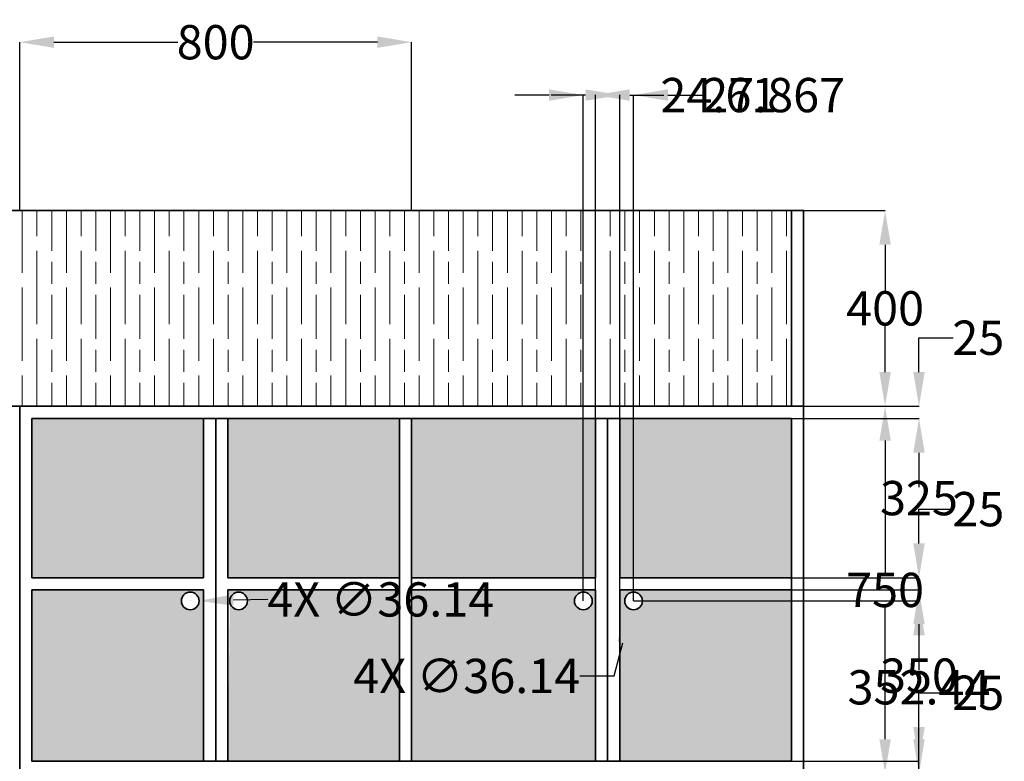
# Model space of a CAD drawing. Units: inches. Extents: x 600 to 5582, y -464 to 3142.
# Tile 9 of 9: x 3385 to 5394, y 1627 to 3142. Entities that reach past the tile are written whole.
import ezdxf

# ---------------------------------------------------------------- set-up
doc = ezdxf.new("R2010")
doc.units = ezdxf.units.IN
doc.header["$MEASUREMENT"] = 0
for name, color, linetype, lineweight in [('A-ANNO-DIMS', 2, 'Continuous', 18), ('A-ELEV', 7, 'Continuous', 35), ('A-ELEV-PATT', 252, 'Continuous', 13)]:
    doc.layers.add(name, color=color, linetype=linetype, lineweight=lineweight)
doc.styles.get("Standard").update_dxf_attribs({"font": 'arial.ttf'})
doc.dimstyles.get("Standard").update_dxf_attribs({"dimtxt": 70, "dimasz": 70, "dimexe": 0.18, "dimexo": 0.0625, "dimgap": 0.09, "dimtad": 0, "dimtih": 1, "dimtoh": 1, "dimdec": 0, "dimzin": 0, "dimdsep": 46, "dimtxsty": 'Standard', "dimcen": 0.09, "dimadec": 0, "dimazin": 0, "dimtfac": 1, "dimtdec": 0, "dimtofl": 0, "dimtmove": 0, "dimatfit": 3, "dimfxl": 1, "dimtolj": 1, "dimtzin": 0, "dimarcsym": 0})

# ---------------------------------------------------------------- blocks, each defined once
blk = doc.blocks.new('*D5')
at = {"layer": 'A-ANNO-DIMS', "color": 0, "lineweight": -2, "transparency": 16777216}
for p, q in [((4984.8, 2352.4), (5151.2, 2352.4)), ((5151, 2282.4), (5151, 2013.3)), ((5151, 1672.4), (5151, 1941.6)), ((4984.8, 1602.4), (5151.2, 1602.4))]:
    blk.add_line(p, q, dxfattribs=at)
at = {"layer": 'A-ANNO-DIMS', "color": 0, "transparency": 16777216}
for points in [[(5139.4, 2282.4), (5162.7, 2282.4), (5151, 2352.4)], [(5139.4, 1672.4), (5162.7, 1672.4), (5151, 1602.4)]]:
    blk.add_solid(points, dxfattribs=at)
at = {"layer": 'Defpoints', "color": 0, "transparency": 16777216}
for p in [(4984.7, 2352.4), (4984.7, 1602.4), (5151, 1602.4)]:
    blk.add_point(p, dxfattribs=at)
at = {"layer": 'A-ANNO-DIMS', "color": 0, "transparency": 16777216, "insert": (5151, 1977.4), "char_height": 70, "attachment_point": 5}
blk.add_mtext('\\A1;750', dxfattribs=at)
blk = doc.blocks.new('*D6')
at = {"layer": 'A-ANNO-DIMS', "color": 0, "lineweight": -2, "transparency": 16777216}
for p, q in [((4984.8, 2752.4), (5151.2, 2752.4)), ((5151, 2682.4), (5151, 2588.3)), ((5151, 2422.4), (5151, 2516.6)), ((4984.8, 2352.4), (5151.2, 2352.4))]:
    blk.add_line(p, q, dxfattribs=at)
at = {"layer": 'A-ANNO-DIMS', "color": 0, "transparency": 16777216}
for points in [[(5139.4, 2682.4), (5162.7, 2682.4), (5151, 2752.4)], [(5139.4, 2422.4), (5162.7, 2422.4), (5151, 2352.4)]]:
    blk.add_solid(points, dxfattribs=at)
at = {"layer": 'Defpoints', "color": 0, "transparency": 16777216}
for p in [(4984.7, 2752.4), (4984.7, 2352.4), (5151, 2352.4)]:
    blk.add_point(p, dxfattribs=at)
at = {"layer": 'A-ANNO-DIMS', "color": 0, "transparency": 16777216, "insert": (5151, 2552.4), "char_height": 70, "attachment_point": 5}
blk.add_mtext('\\A1;400', dxfattribs=at)
blk = doc.blocks.new('*D9')
at = {"layer": 'A-ANNO-DIMS', "color": 0, "lineweight": -2, "transparency": 16777216}
for p, q in [((3384.7, 2752.5), (3384.7, 3096.1)), ((3454.7, 3095.9), (3707.4, 3095.9)), ((4114.7, 3095.9), (3862.1, 3095.9)), ((4184.7, 2752.5), (4184.7, 3096.1))]:
    blk.add_line(p, q, dxfattribs=at)
at = {"layer": 'A-ANNO-DIMS', "color": 0, "transparency": 16777216}
for points in [[(3454.7, 3107.6), (3454.7, 3084.3), (3384.7, 3095.9)], [(4114.7, 3107.6), (4114.7, 3084.3), (4184.7, 3095.9)]]:
    blk.add_solid(points, dxfattribs=at)
at = {"layer": 'Defpoints', "color": 0, "transparency": 16777216}
for p in [(4184.7, 3095.9), (3384.7, 2752.4), (4184.7, 2752.4)]:
    blk.add_point(p, dxfattribs=at)
at = {"layer": 'A-ANNO-DIMS', "color": 0, "transparency": 16777216, "insert": (3784.7, 3095.9), "char_height": 70, "attachment_point": 5}
blk.add_mtext('\\A1;800', dxfattribs=at)
blk = doc.blocks.new('*D35')
at = {"layer": 'A-ANNO-DIMS', "color": 0, "lineweight": -2, "transparency": 16777216}
for p, q in [((5220.2, 1697.4), (5220.2, 1767.4)), ((5220.2, 1767.4), (5290.2, 1767.4)), ((4959.8, 1627.4), (5220.4, 1627.4)), ((4984.8, 1602.4), (5220.4, 1602.4)), ((5220.2, 1532.4), (5220.2, 1462.4))]:
    blk.add_line(p, q, dxfattribs=at)
at = {"layer": 'A-ANNO-DIMS', "color": 0, "transparency": 16777216}
for points in [[(5208.6, 1697.4), (5231.9, 1697.4), (5220.2, 1627.4)], [(5208.6, 1532.4), (5231.9, 1532.4), (5220.2, 1602.4)]]:
    blk.add_solid(points, dxfattribs=at)
at = {"layer": 'Defpoints', "color": 0, "transparency": 16777216}
for p in [(4959.7, 1627.4), (5220.2, 1627.4), (4984.7, 1602.4)]:
    blk.add_point(p, dxfattribs=at)
at = {"layer": 'A-ANNO-DIMS', "color": 0, "transparency": 16777216, "insert": (5341.3, 1767.4), "char_height": 70, "attachment_point": 5}
blk.add_mtext('\\A1;25', dxfattribs=at)
blk = doc.blocks.new('*D36')
at = {"layer": 'A-ANNO-DIMS', "color": 0, "lineweight": -2, "transparency": 16777216}
for p, q in [((4959.8, 1977.4), (5220.4, 1977.4)), ((5220.2, 1907.4), (5220.2, 1838.3)), ((5220.2, 1697.4), (5220.2, 1766.6)), ((4959.8, 1627.4), (5220.4, 1627.4))]:
    blk.add_line(p, q, dxfattribs=at)
at = {"layer": 'A-ANNO-DIMS', "color": 0, "transparency": 16777216}
for points in [[(5208.6, 1907.4), (5231.9, 1907.4), (5220.2, 1977.4)], [(5208.6, 1697.4), (5231.9, 1697.4), (5220.2, 1627.4)]]:
    blk.add_solid(points, dxfattribs=at)
at = {"layer": 'Defpoints', "color": 0, "transparency": 16777216}
for p in [(4959.7, 1977.4), (5220.2, 1977.4), (4959.7, 1627.4)]:
    blk.add_point(p, dxfattribs=at)
at = {"layer": 'A-ANNO-DIMS', "color": 0, "transparency": 16777216, "insert": (5220.2, 1802.4), "char_height": 70, "attachment_point": 5}
blk.add_mtext('\\A1;350', dxfattribs=at)
blk = doc.blocks.new('*D37')
at = {"layer": 'A-ANNO-DIMS', "color": 0, "lineweight": -2, "transparency": 16777216}
for p, q in [((5220.2, 2072.4), (5220.2, 2142.4)), ((5220.2, 2142.4), (5290.2, 2142.4)), ((4959.8, 2002.4), (5220.4, 2002.4)), ((4959.8, 1977.4), (5220.4, 1977.4)), ((5220.2, 1907.4), (5220.2, 1837.4))]:
    blk.add_line(p, q, dxfattribs=at)
at = {"layer": 'A-ANNO-DIMS', "color": 0, "transparency": 16777216}
for points in [[(5208.6, 2072.4), (5231.9, 2072.4), (5220.2, 2002.4)], [(5208.6, 1907.4), (5231.9, 1907.4), (5220.2, 1977.4)]]:
    blk.add_solid(points, dxfattribs=at)
at = {"layer": 'Defpoints', "color": 0, "transparency": 16777216}
for p in [(4959.7, 2002.4), (5220.2, 2002.4), (4959.7, 1977.4)]:
    blk.add_point(p, dxfattribs=at)
at = {"layer": 'A-ANNO-DIMS', "color": 0, "transparency": 16777216, "insert": (5341.3, 2142.4), "char_height": 70, "attachment_point": 5}
blk.add_mtext('\\A1;25', dxfattribs=at)
blk = doc.blocks.new('*D38')
at = {"layer": 'A-ANNO-DIMS', "color": 0, "lineweight": -2, "transparency": 16777216}
for p, q in [((4959.8, 2327.4), (5220.4, 2327.4)), ((5220.2, 2257.4), (5220.2, 2200.8)), ((5220.2, 2072.4), (5220.2, 2129.1)), ((4959.8, 2002.4), (5220.4, 2002.4))]:
    blk.add_line(p, q, dxfattribs=at)
at = {"layer": 'A-ANNO-DIMS', "color": 0, "transparency": 16777216}
for points in [[(5208.6, 2257.4), (5231.9, 2257.4), (5220.2, 2327.4)], [(5208.6, 2072.4), (5231.9, 2072.4), (5220.2, 2002.4)]]:
    blk.add_solid(points, dxfattribs=at)
at = {"layer": 'Defpoints', "color": 0, "transparency": 16777216}
for p in [(4959.7, 2327.4), (5220.2, 2327.4), (4959.7, 2002.4)]:
    blk.add_point(p, dxfattribs=at)
at = {"layer": 'A-ANNO-DIMS', "color": 0, "transparency": 16777216, "insert": (5220.2, 2164.9), "char_height": 70, "attachment_point": 5}
blk.add_mtext('\\A1;325', dxfattribs=at)
blk = doc.blocks.new('*D39')
at = {"layer": 'A-ANNO-DIMS', "color": 0, "lineweight": -2, "transparency": 16777216}
for p, q in [((5220.2, 2422.4), (5220.2, 2492.4)), ((5220.2, 2492.4), (5290.2, 2492.4)), ((4984.8, 2352.4), (5220.4, 2352.4)), ((4959.8, 2327.4), (5220.4, 2327.4)), ((5220.2, 2257.4), (5220.2, 2187.4))]:
    blk.add_line(p, q, dxfattribs=at)
at = {"layer": 'A-ANNO-DIMS', "color": 0, "transparency": 16777216}
for points in [[(5208.6, 2422.4), (5231.9, 2422.4), (5220.2, 2352.4)], [(5208.6, 2257.4), (5231.9, 2257.4), (5220.2, 2327.4)]]:
    blk.add_solid(points, dxfattribs=at)
at = {"layer": 'Defpoints', "color": 0, "transparency": 16777216}
for p in [(4984.7, 2352.4), (5220.2, 2352.4), (4959.7, 2327.4)]:
    blk.add_point(p, dxfattribs=at)
at = {"layer": 'A-ANNO-DIMS', "color": 0, "transparency": 16777216, "insert": (5341.3, 2492.4), "char_height": 70, "attachment_point": 5}
blk.add_mtext('\\A1;25', dxfattribs=at)
blk = doc.blocks.new('*D58')
at = {"layer": 'A-ANNO-DIMS', "color": 0, "lineweight": -2, "transparency": 16777216}
for p, q in [((3732.7, 1954.9), (3732.9, 1954.9)), ((3732.8, 1954.8), (3732.8, 1954.9)), ((3890.9, 1958), (3820.9, 1956.6))]:
    blk.add_line(p, q, dxfattribs=at)
at = {"layer": 'A-ANNO-DIMS', "color": 0, "transparency": 16777216}
blk.add_solid([(3820.6, 1968.3), (3821.1, 1944.9), (3750.9, 1955.2)], dxfattribs=at)
at = {"layer": 'Defpoints', "color": 0, "transparency": 16777216}
for p in [(3714.8, 1954.5), (3750.9, 1955.2)]:
    blk.add_point(p, dxfattribs=at)
at = {"layer": 'A-ANNO-DIMS', "color": 0, "transparency": 16777216, "insert": (4121.7, 1958), "char_height": 70, "attachment_point": 5}
blk.add_mtext('\\A1;4X ∅36.14', dxfattribs=at)
blk = doc.blocks.new('*D60')
at = {"layer": 'A-ANNO-DIMS', "color": 0, "lineweight": -2, "transparency": 16777216}
for p, q in [((4539.7, 2987.9), (4469.7, 2987.9)), ((4609.7, 1977.5), (4609.7, 2988.1)), ((4637.6, 1954.9), (4637.6, 2988.1)), ((4707.6, 2987.9), (4777.6, 2987.9))]:
    blk.add_line(p, q, dxfattribs=at)
at = {"layer": 'A-ANNO-DIMS', "color": 0, "transparency": 16777216}
for points in [[(4539.7, 2999.6), (4539.7, 2976.3), (4609.7, 2987.9)], [(4707.6, 2999.6), (4707.6, 2976.3), (4637.6, 2987.9)]]:
    blk.add_solid(points, dxfattribs=at)
at = {"layer": 'Defpoints', "color": 0, "transparency": 16777216}
for p in [(4637.6, 2987.9), (4609.7, 1977.4), (4637.6, 1954.9)]:
    blk.add_point(p, dxfattribs=at)
at = {"layer": 'A-ANNO-DIMS', "color": 0, "transparency": 16777216, "insert": (4923.6, 2987.9), "char_height": 70, "attachment_point": 5}
blk.add_mtext('\\A1;27.867', dxfattribs=at)
blk = doc.blocks.new('*D61')
at = {"layer": 'A-ANNO-DIMS', "color": 0, "lineweight": -2, "transparency": 16777216}
for p, q in [((4637.7, 1954.9), (5220.4, 1954.9)), ((5220.2, 1884.9), (5220.2, 1814.5)), ((5220.2, 1672.4), (5220.2, 1742.8)), ((4984.8, 1602.4), (5220.4, 1602.4))]:
    blk.add_line(p, q, dxfattribs=at)
at = {"layer": 'A-ANNO-DIMS', "color": 0, "transparency": 16777216}
for points in [[(5208.6, 1884.9), (5231.9, 1884.9), (5220.2, 1954.9)], [(5208.6, 1672.4), (5231.9, 1672.4), (5220.2, 1602.4)]]:
    blk.add_solid(points, dxfattribs=at)
at = {"layer": 'Defpoints', "color": 0, "transparency": 16777216}
for p in [(4637.6, 1954.9), (5220.2, 1954.9), (4984.7, 1602.4)]:
    blk.add_point(p, dxfattribs=at)
at = {"layer": 'A-ANNO-DIMS', "color": 0, "transparency": 16777216, "insert": (5220.2, 1778.6), "char_height": 70, "attachment_point": 5}
blk.add_mtext('\\A1;352.44', dxfattribs=at)
blk = doc.blocks.new('*D62')
at = {"layer": 'A-ANNO-DIMS', "color": 0, "lineweight": -2, "transparency": 16777216}
for p, q in [((4465.1, 2987.9), (4395.1, 2987.9)), ((4535.1, 1954.9), (4535.1, 2988.1)), ((4559.7, 1977.5), (4559.7, 2988.1)), ((4629.7, 2987.9), (4699.7, 2987.9))]:
    blk.add_line(p, q, dxfattribs=at)
at = {"layer": 'A-ANNO-DIMS', "color": 0, "transparency": 16777216}
for points in [[(4465.1, 2999.6), (4465.1, 2976.3), (4535.1, 2987.9)], [(4629.7, 2999.6), (4629.7, 2976.3), (4559.7, 2987.9)]]:
    blk.add_solid(points, dxfattribs=at)
at = {"layer": 'Defpoints', "color": 0, "transparency": 16777216}
for p in [(4559.7, 2987.9), (4559.7, 1977.4), (4535.1, 1954.9)]:
    blk.add_point(p, dxfattribs=at)
at = {"layer": 'A-ANNO-DIMS', "color": 0, "transparency": 16777216, "insert": (4811.8, 2987.9), "char_height": 70, "attachment_point": 5}
blk.add_mtext('\\A1;24.61', dxfattribs=at)
blk = doc.blocks.new('*D64')
at = {"layer": 'A-ANNO-DIMS', "color": 0, "lineweight": -2, "transparency": 16777216}
for p, q in [((3384.7, 1680.8), (3384.7, -233.3)), ((3356.6, 1655.8), (3356.6, -233.3)), ((3286.6, -233.1), (3216.6, -233.1)), ((3454.7, -233.1), (3524.7, -233.1))]:
    blk.add_line(p, q, dxfattribs=at)
at = {"layer": 'A-ANNO-DIMS', "color": 0, "transparency": 16777216}
for points in [[(3286.6, -221.4), (3286.6, -244.7), (3356.6, -233.1)], [(3454.7, -221.4), (3454.7, -244.7), (3384.7, -233.1)]]:
    blk.add_solid(points, dxfattribs=at)
at = {"layer": 'Defpoints', "color": 0, "transparency": 16777216}
for p in [(3384.7, 1680.8), (3356.6, 1655.8), (3384.7, -233.1)]:
    blk.add_point(p, dxfattribs=at)
at = {"layer": 'A-ANNO-DIMS', "color": 0, "transparency": 16777216, "insert": (3643.5, -233.1), "char_height": 70, "attachment_point": 5}
blk.add_mtext('\\A1;28.17', dxfattribs=at)
blk = doc.blocks.new('*D99')
at = {"layer": 'A-ANNO-DIMS', "color": 0, "lineweight": -2, "transparency": 16777216}
for p, q in [((5220.2, 1603.5), (5220.2, 1673.5)), ((2271, 1533.5), (5220.4, 1533.5)), ((2273, 1464.8), (5220.4, 1464.8)), ((5220.2, 1394.8), (5220.2, 1324.8)), ((5220.2, 1324.8), (5150.2, 1324.8))]:
    blk.add_line(p, q, dxfattribs=at)
at = {"layer": 'A-ANNO-DIMS', "color": 0, "transparency": 16777216}
for points in [[(5208.6, 1603.5), (5231.9, 1603.5), (5220.2, 1533.5)], [(5208.6, 1394.8), (5231.9, 1394.8), (5220.2, 1464.8)]]:
    blk.add_solid(points, dxfattribs=at)
at = {"layer": 'Defpoints', "color": 0, "transparency": 16777216}
for p in [(2271, 1533.5), (2272.9, 1464.8), (5220.2, 1464.8)]:
    blk.add_point(p, dxfattribs=at)
at = {"layer": 'A-ANNO-DIMS', "color": 0, "transparency": 16777216, "insert": (5038.6, 1324.8), "char_height": 70, "attachment_point": 5}
blk.add_mtext('\\A1;68.71', dxfattribs=at)
blk = doc.blocks.new('*D102')
at = {"layer": 'A-ANNO-DIMS', "color": 0, "lineweight": -2, "transparency": 16777216}
for p, q in [((4637.5, 1954.9), (4637.7, 1954.9)), ((4637.6, 1954.8), (4637.6, 1954.9)), ((4598.1, 1801.8), (4615.6, 1869.6)), ((4528.1, 1801.8), (4598.1, 1801.8))]:
    blk.add_line(p, q, dxfattribs=at)
at = {"layer": 'A-ANNO-DIMS', "color": 0, "transparency": 16777216}
blk.add_solid([(4604.3, 1872.5), (4626.9, 1866.7), (4633.1, 1937.4)], dxfattribs=at)
at = {"layer": 'Defpoints', "color": 0, "transparency": 16777216}
for p in [(4642.1, 1972.4), (4633.1, 1937.4)]:
    blk.add_point(p, dxfattribs=at)
at = {"layer": 'A-ANNO-DIMS', "color": 0, "transparency": 16777216, "insert": (4297.2, 1801.8), "char_height": 70, "attachment_point": 5}
blk.add_mtext('\\A1;4X ∅36.14', dxfattribs=at)

msp = doc.modelspace()

# ---------------------------------------------------------------- hatches: boundary and pattern name
at = {"layer": 'A-ELEV-PATT'}
h = msp.add_hatch(dxfattribs=at)
h.set_pattern_fill('GOST_WOOD', color=256, scale=15)
h.set_pattern_definition([(90, (0, 0), (90, -6e-15), [150, -30]), (90, (30, -30), (90, -6e-15), [90, -22.5, 45, -22.5]), (90, (60, -75), (90, -6e-15), [150, -30])])
h.paths.add_polyline_path([(4959.7485, 2752.4212), (1409.7485, 2752.4212), (1409.7485, 2352.4212), (1784.7485, 2352.4212), (4959.7485, 2352.4212)])
h.paths.add_polyline_path([(3384.7485, 1002.4212), (2584.7485, 1002.4212), (2584.7485, 777.4212), (3384.7485, 777.4212)])
h.paths.add_polyline_path([(3384.7485, 777.4212), (2584.7485, 777.4212), (2584.7485, 552.4212), (3384.7485, 552.4212)])
h.paths.add_polyline_path([(3384.7485, 512.4212), (2584.7485, 512.4212), (2584.7485, 102.4212), (3384.7485, 102.4212)])
h = msp.add_hatch(dxfattribs=at)
h.set_pattern_fill('CROSS', color=256, scale=100)
h.paths.add_polyline_path([(1759.7485, 2327.4212), (1409.7485, 2327.4212), (1409.7485, 1967.4212), (1759.7485, 1967.4212)])
h.paths.add_polyline_path([(1759.7485, 1952.4212), (1409.7485, 1952.4212), (1409.7485, 1567.4212), (1759.7485, 1567.4212)])
h.paths.add_polyline_path([(1759.7485, 1552.4212), (1409.7485, 1552.4212), (1409.7485, 1167.4212), (1759.7485, 1167.4212)])
h.paths.add_polyline_path([(1759.7485, 1152.4212), (1409.7485, 1152.4212), (1409.7485, 767.4212), (1759.7485, 767.4212)])
h.paths.add_polyline_path([(1759.7485, 752.4212), (1409.7485, 752.4212), (1409.7485, 367.4212), (1759.7485, 367.4212)])
h.paths.add_polyline_path([(1759.7485, 352.4212), (1409.7485, 352.4212), (1409.7485, 142.4212), (1759.7485, 142.4212)])
h.paths.add_polyline_path([(3759.7485, 1977.4212), (3409.7485, 1977.4212), (3409.7485, 1627.4212), (3759.7485, 1627.4212)])
h.paths.add_polyline_path([(3714.7508, 1954.858, -1), (3750.8891, 1954.858, -1)], flags=16)
h.paths.add_polyline_path([(3759.7485, 2327.4212), (3409.7485, 2327.4212), (3409.7485, 2002.4212), (3759.7485, 2002.4212)])
h.paths.add_polyline_path([(4159.7485, 2327.4212), (3809.7485, 2327.4212), (3809.7485, 2002.4212), (4159.7485, 2002.4212)])
h.paths.add_polyline_path([(4159.7485, 1977.4212), (3809.7485, 1977.4212), (3813.5467, 1954.858, -1), (3849.685, 1954.858, -1), (3813.5467, 1954.858), (3809.7485, 1627.4212), (4159.7485, 1627.4212)])
h.paths.add_polyline_path([(4559.7485, 2327.4212), (4184.7485, 2327.4212), (4184.7485, 2002.4212), (4559.7485, 2002.4212)])
h.paths.add_polyline_path([(4559.7485, 1977.4212), (4184.7485, 1977.4212), (4184.7485, 1627.4212), (4559.7485, 1627.4212)])
h.paths.add_polyline_path([(4517.0704, 1954.858, -1), (4553.2087, 1954.858, -1)], flags=16)
h.paths.add_polyline_path([(4959.7485, 2327.4212), (4609.7485, 2327.4212), (4609.7485, 2002.4212), (4959.7485, 2002.4212)])
h.paths.add_polyline_path([(4959.7485, 1977.4212), (4609.7485, 1977.4212), (4609.7485, 1627.4212), (4959.7485, 1627.4212)])
h.paths.add_polyline_path([(4619.5464, 1954.858, -1), (4655.6847, 1954.858, -1)], flags=16)

# ---------------------------------------------------------------- linework, layer by layer
at = {"layer": 'A-ELEV'}
for p, q in [((4959.7485, 2352.4212), (4959.7485, 2752.4212)), ((4984.7485, 2352.4212), (1384.7485, 2352.4212)), ((4184.7485, 2352.4212), (4584.7485, 2352.4212)), ((3784.7485, 2327.4212), (3784.7485, 1627.4212)), ((4159.7485, 1627.4212), (4159.7485, 2327.4212)), ((4184.7485, 1627.4212), (4184.7485, 2327.4212)), ((4584.7485, 2327.4212), (4584.7485, 1627.4212))]:
    msp.add_line(p, q, dxfattribs=at)
msp.add_lwpolyline([(4984.7485, 2.4212), (4984.7485, 2752.4212), (1384.7485, 2752.4212), (1384.7485, 2.4212)], close=True, dxfattribs=at)
for points in [[(4984.7485, 1602.4212), (3384.7485, 1602.4212), (3384.7485, 2352.4212), (3784.7485, 2352.4212)], [(3759.7485, 2327.4212), (3759.7485, 2002.4212), (3409.7485, 2002.4212), (3409.7485, 2327.4212), (4959.7485, 2327.4212), (4959.7485, 1627.4212), (3409.7485, 1627.4212), (3409.7485, 1977.4212), (3759.7485, 1977.4212), (3759.7485, 1627.4212)], [(3809.7485, 2327.4212), (3809.7485, 2002.4212), (4159.7485, 2002.4212)], [(4559.7485, 2327.4212), (4559.7485, 2002.4212), (4184.7485, 2002.4212)], [(4609.7485, 2327.4212), (4609.7485, 2002.4212), (4959.7485, 2002.4212)], [(4159.7485, 1977.4212), (3809.7485, 1977.4212), (3809.7485, 1627.4212)], [(4184.7485, 1977.4212), (4559.7485, 1977.4212), (4559.7485, 1627.4212)], [(4959.7485, 1977.4212), (4609.7485, 1977.4212), (4609.7485, 1627.4212)]]:
    msp.add_lwpolyline(points, dxfattribs=at)
for centre in [(3732.8199, 1954.858), (3831.6158, 1954.858), (4535.1396, 1954.858), (4637.6155, 1954.858)]:
    msp.add_circle(centre, 18.0692, dxfattribs=at)

# ---------------------------------------------------------------- dimensions: what is measured, and where the dimension line sits
at = {"layer": 'A-ANNO-DIMS'}
for base, p1, p2, override, picture, middle in [((4184.7485, 3095.9369), (3384.7485, 2752.4212), (4184.7485, 2752.4212), {"dimclrd": 0, "dimclre": 0, "dimclrt": 0}, '*D9', (3784.7485, 3095.9369)), ((4559.7485, 2987.9212), (4535.1396, 1954.858), (4559.7485, 1977.4212), {"dimdec": 2, "dimlfac": 1, "dimrnd": 0, "dimzin": 0, "dimdsep": 46, "dimlunit": 2}, '*D62', (4811.786, 2987.9212)), ((4637.6155, 2987.9212), (4609.7485, 1977.4212), (4637.6155, 1954.858), {"dimdec": 3, "dimlfac": 1, "dimrnd": 0, "dimzin": 0, "dimdsep": 46, "dimlunit": 2}, '*D60', (4923.6025, 2987.9212)), ((3384.7485, -233.0788), (3356.5781, 1655.8271), (3384.7485, 1680.8271), {"dimdec": 2, "dimlfac": 1, "dimrnd": 0, "dimzin": 0, "dimdsep": 46, "dimlunit": 2}, '*D64', (3643.5424, -233.0788))]:
    dim = msp.add_linear_dim(base=base, p1=p1, p2=p2, dimstyle='Standard', override=override, dxfattribs=at)
    dim.commit()
    dim.dimension.update_dxf_attribs({"geometry": picture, "text_midpoint": middle})
for base, p1, p2, override, picture, middle in [((5151.032, 2352.4212), (4984.7485, 2752.4212), (4984.7485, 2352.4212), {"dimclrd": 0, "dimclre": 0, "dimclrt": 0}, '*D6', (5151.032, 2552.4212)), ((5220.2485, 2352.4212), (4959.7485, 2327.4212), (4984.7485, 2352.4212), {"dimdec": 0, "dimlfac": 1, "dimrnd": 0, "dimzin": 0, "dimdsep": 46, "dimlunit": 2}, '*D39', (5341.3344, 2492.4212)), ((5151.032, 1602.4212), (4984.7485, 2352.4212), (4984.7485, 1602.4212), {"dimclrd": 0, "dimclre": 0, "dimclrt": 0}, '*D5', (5151.032, 1977.4212)), ((5220.2485, 2327.4212), (4959.7485, 2002.4212), (4959.7485, 2327.4212), {"dimdec": 0, "dimlfac": 1, "dimrnd": 0, "dimzin": 0, "dimdsep": 46, "dimlunit": 2}, '*D38', (5220.2485, 2164.9212)), ((5220.2485, 2002.4212), (4959.7485, 1977.4212), (4959.7485, 2002.4212), {"dimdec": 0, "dimlfac": 1, "dimrnd": 0, "dimzin": 0, "dimdsep": 46, "dimlunit": 2}, '*D37', (5341.3344, 2142.4212)), ((5220.2485, 1977.4212), (4959.7485, 1627.4212), (4959.7485, 1977.4212), {"dimdec": 0, "dimlfac": 1, "dimrnd": 0, "dimzin": 0, "dimdsep": 46, "dimlunit": 2}, '*D36', (5220.2485, 1802.4212)), ((5220.2485, 1954.858), (4984.7485, 1602.4212), (4637.6155, 1954.858), {"dimdec": 2, "dimlfac": 1, "dimrnd": 0, "dimzin": 0, "dimdsep": 46, "dimlunit": 2}, '*D61', (5220.2485, 1778.6396)), ((5220.2485, 1627.4212), (4984.7485, 1602.4212), (4959.7485, 1627.4212), {"dimdec": 0, "dimlfac": 1, "dimrnd": 0, "dimzin": 0, "dimdsep": 46, "dimlunit": 2}, '*D35', (5341.3344, 1767.4212)), ((5220.2485, 1464.7817), (2270.9593, 1533.4874), (2272.9025, 1464.7817), {"dimdec": 2, "dimlfac": 1, "dimrnd": 0, "dimzin": 0, "dimdsep": 46, "dimlunit": 2}, '*D99', (5038.6169, 1324.7817))]:
    dim = msp.add_linear_dim(base=base, p1=p1, p2=p2, angle=90, dimstyle='Standard', override=override, dxfattribs=at)
    dim.commit()
    dim.dimension.update_dxf_attribs({"geometry": picture, "text_midpoint": middle})
for p1, p2, picture, middle in [((3714.7543, 1954.5007), (3750.8855, 1955.2153), '*D58', (3890.8582, 1957.9836)), ((4642.1371, 1972.3523), (4633.094, 1937.3637), '*D102', (4297.1764, 1801.8178))]:
    dim = msp.add_diameter_dim_2p(p1=p1, p2=p2, text='4X <>', dimstyle='Standard', override={"dimdec": 2, "dimlfac": 1, "dimrnd": 0, "dimzin": 0, "dimdsep": 46, "dimlunit": 2}, dxfattribs=at)
    dim.commit()
    dim.dimension.update_dxf_attribs({"geometry": picture, "text_midpoint": middle, "dimtype": 163})

doc.saveas('drawing.dxf')
